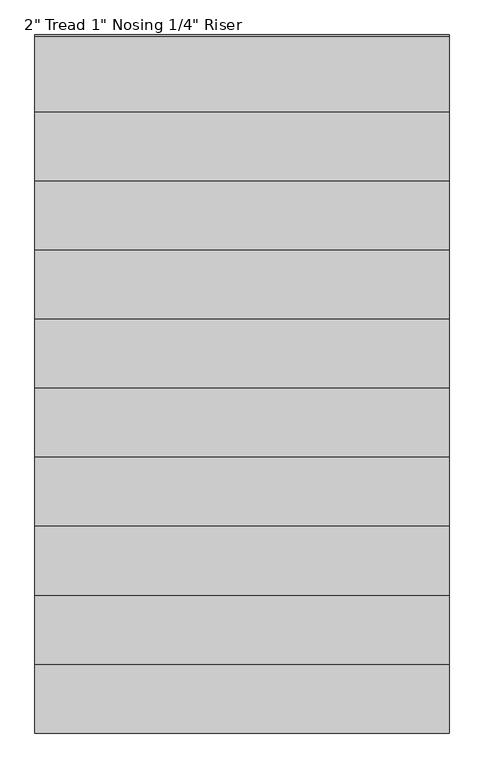
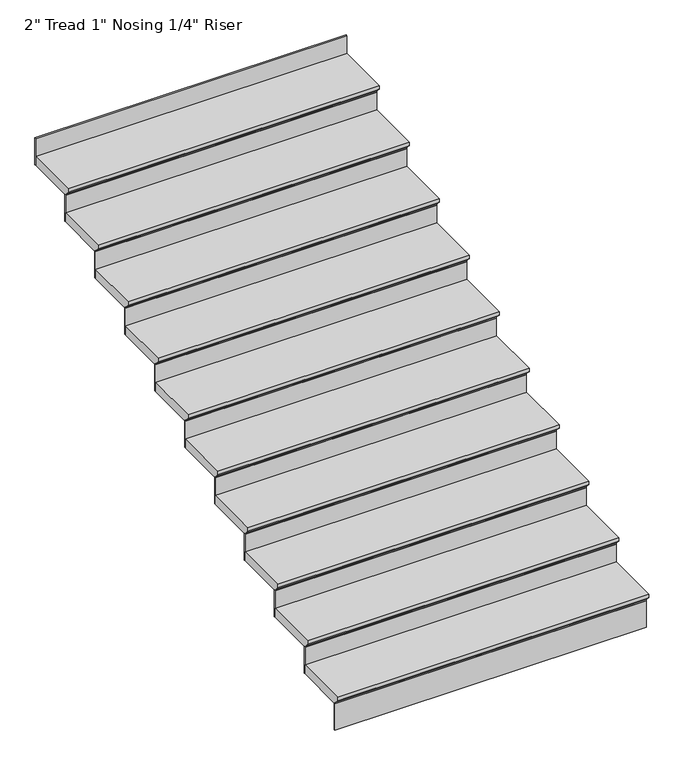
"""IFC4 building model written with IfcOpenShell, lengths in millimetres: stair flight geometry."""

from ifc_helpers import new_model, si_unit, frame, origin, place, context, project, spatial, polyline, outline, extrude, source, transform, mapped, element, save


def stair_flight_a36623a9(model_context):
    return source(origin(), model_context, "Body", "SweptSolid", [
        extrude(outline(polyline([(30952.1590238, 2286.0), (31256.9590238, 2286.0), (31256.9590238, 2235.2), (30977.5590238, 2235.2), (30977.5590238, 2241.55), (30952.1590238, 2266.95), (30952.1590238, 2286.0)])), frame((55546.5312819, 0.0, 0.0), z_axis=(1.0, 0.0, 0.0), x_axis=(0.0, 1.0, 0.0)), (0.0, 0.0, 1.0), 1676.4),
        extrude(outline(polyline([(57222.9312819, 30983.9090238), (57222.9312819, 30977.5590238), (55546.5312819, 30977.5590238), (55546.5312819, 30983.9090238), (57222.9312819, 30983.9090238)])), frame((0.0, 0.0, 2082.8), z_axis=(0.0, 0.0, 1.0), x_axis=(1.0, 0.0, 0.0)), (0.0, 0.0, 1.0), 152.4),
        extrude(outline(polyline([(57222.9312819, 31263.3090238), (57222.9312819, 31256.9590238), (55546.5312819, 31256.9590238), (55546.5312819, 31263.3090238), (57222.9312819, 31263.3090238)])), frame((0.0, 0.0, 2235.2), z_axis=(0.0, 0.0, 1.0), x_axis=(1.0, 0.0, 0.0)), (0.0, 0.0, 1.0), 152.4),
        extrude(outline(polyline([(31231.5590238, 2438.4), (31536.3590238, 2438.4), (31536.3590238, 2387.6), (31256.9590238, 2387.6), (31256.9590238, 2393.95), (31231.5590238, 2419.35), (31231.5590238, 2438.4)])), frame((55546.5312819, 0.0, 0.0), z_axis=(1.0, 0.0, 0.0), x_axis=(0.0, 1.0, 0.0)), (0.0, 0.0, 1.0), 1676.4),
        extrude(outline(polyline([(57222.9312819, 31542.7090238), (57222.9312819, 31536.3590238), (55546.5312819, 31536.3590238), (55546.5312819, 31542.7090238), (57222.9312819, 31542.7090238)])), frame((0.0, 0.0, 2387.6), z_axis=(0.0, 0.0, 1.0), x_axis=(1.0, 0.0, 0.0)), (0.0, 0.0, 1.0), 152.4),
        extrude(outline(polyline([(31510.9590238, 2590.8), (31815.7590238, 2590.8), (31815.7590238, 2540.0), (31536.3590238, 2540.0), (31536.3590238, 2546.35), (31510.9590238, 2571.75), (31510.9590238, 2590.8)])), frame((55546.5312819, 0.0, 0.0), z_axis=(1.0, 0.0, 0.0), x_axis=(0.0, 1.0, 0.0)), (0.0, 0.0, 1.0), 1676.4),
        extrude(outline(polyline([(57222.9312819, 31822.1090238), (57222.9312819, 31815.7590238), (55546.5312819, 31815.7590238), (55546.5312819, 31822.1090238), (57222.9312819, 31822.1090238)])), frame((0.0, 0.0, 2540.0), z_axis=(0.0, 0.0, 1.0), x_axis=(1.0, 0.0, 0.0)), (0.0, 0.0, 1.0), 152.4),
        extrude(outline(polyline([(31790.3590238, 2743.2), (32095.1590238, 2743.2), (32095.1590238, 2692.4), (31815.7590238, 2692.4), (31815.7590238, 2698.75), (31790.3590238, 2724.15), (31790.3590238, 2743.2)])), frame((55546.5312819, 0.0, 0.0), z_axis=(1.0, 0.0, 0.0), x_axis=(0.0, 1.0, 0.0)), (0.0, 0.0, 1.0), 1676.4),
        extrude(outline(polyline([(57222.9312819, 32101.5090238), (57222.9312819, 32095.1590238), (55546.5312819, 32095.1590238), (55546.5312819, 32101.5090238), (57222.9312819, 32101.5090238)])), frame((0.0, 0.0, 2692.4), z_axis=(0.0, 0.0, 1.0), x_axis=(1.0, 0.0, 0.0)), (0.0, 0.0, 1.0), 152.4),
        extrude(outline(polyline([(32069.7590238, 2895.6), (32374.5590238, 2895.6), (32374.5590238, 2844.8), (32095.1590238, 2844.8), (32095.1590238, 2851.15), (32069.7590238, 2876.55), (32069.7590238, 2895.6)])), frame((55546.5312819, 0.0, 0.0), z_axis=(1.0, 0.0, 0.0), x_axis=(0.0, 1.0, 0.0)), (0.0, 0.0, 1.0), 1676.4),
        extrude(outline(polyline([(57222.9312819, 32380.9090238), (57222.9312819, 32374.5590238), (55546.5312819, 32374.5590238), (55546.5312819, 32380.9090238), (57222.9312819, 32380.9090238)])), frame((0.0, 0.0, 2844.8), z_axis=(0.0, 0.0, 1.0), x_axis=(1.0, 0.0, 0.0)), (0.0, 0.0, 1.0), 152.4),
        extrude(outline(polyline([(32349.1590238, 3048.0), (32653.9590238, 3048.0), (32653.9590238, 2997.2), (32374.5590238, 2997.2), (32374.5590238, 3003.55), (32349.1590238, 3028.95), (32349.1590238, 3048.0)])), frame((55546.5312819, 0.0, 0.0), z_axis=(1.0, 0.0, 0.0), x_axis=(0.0, 1.0, 0.0)), (0.0, 0.0, 1.0), 1676.4),
        extrude(outline(polyline([(57222.9312819, 32660.3090238), (57222.9312819, 32653.9590238), (55546.5312819, 32653.9590238), (55546.5312819, 32660.3090238), (57222.9312819, 32660.3090238)])), frame((0.0, 0.0, 2997.2), z_axis=(0.0, 0.0, 1.0), x_axis=(1.0, 0.0, 0.0)), (0.0, 0.0, 1.0), 152.4),
        extrude(outline(polyline([(32628.5590238, 3200.4), (32933.3590238, 3200.4), (32933.3590238, 3149.6), (32653.9590238, 3149.6), (32653.9590238, 3155.95), (32628.5590238, 3181.35), (32628.5590238, 3200.4)])), frame((55546.5312819, 0.0, 0.0), z_axis=(1.0, 0.0, 0.0), x_axis=(0.0, 1.0, 0.0)), (0.0, 0.0, 1.0), 1676.4),
        extrude(outline(polyline([(57222.9312819, 32939.7090238), (57222.9312819, 32933.3590238), (55546.5312819, 32933.3590238), (55546.5312819, 32939.7090238), (57222.9312819, 32939.7090238)])), frame((0.0, 0.0, 3149.6), z_axis=(0.0, 0.0, 1.0), x_axis=(1.0, 0.0, 0.0)), (0.0, 0.0, 1.0), 152.4),
        extrude(outline(polyline([(32907.9590238, 3352.8), (33212.7590238, 3352.8), (33212.7590238, 3302.0), (32933.3590238, 3302.0), (32933.3590238, 3308.35), (32907.9590238, 3333.75), (32907.9590238, 3352.8)])), frame((55546.5312819, 0.0, 0.0), z_axis=(1.0, 0.0, 0.0), x_axis=(0.0, 1.0, 0.0)), (0.0, 0.0, 1.0), 1676.4),
        extrude(outline(polyline([(57222.9312819, 33219.1090238), (57222.9312819, 33212.7590238), (55546.5312819, 33212.7590238), (55546.5312819, 33219.1090238), (57222.9312819, 33219.1090238)])), frame((0.0, 0.0, 3302.0), z_axis=(0.0, 0.0, 1.0), x_axis=(1.0, 0.0, 0.0)), (0.0, 0.0, 1.0), 152.4),
        extrude(outline(polyline([(33187.3590238, 3505.2), (33492.1590238, 3505.2), (33492.1590238, 3454.4), (33212.7590238, 3454.4), (33212.7590238, 3460.75), (33187.3590238, 3486.15), (33187.3590238, 3505.2)])), frame((55546.5312819, 0.0, 0.0), z_axis=(1.0, 0.0, 0.0), x_axis=(0.0, 1.0, 0.0)), (0.0, 0.0, 1.0), 1676.4),
        extrude(outline(polyline([(57222.9312819, 33498.5090238), (57222.9312819, 33492.1590238), (55546.5312819, 33492.1590238), (55546.5312819, 33498.5090238), (57222.9312819, 33498.5090238)])), frame((0.0, 0.0, 3454.4), z_axis=(0.0, 0.0, 1.0), x_axis=(1.0, 0.0, 0.0)), (0.0, 0.0, 1.0), 152.4),
        extrude(outline(polyline([(57222.9312819, 33777.9090238), (57222.9312819, 33771.5590238), (55546.5312819, 33771.5590238), (55546.5312819, 33777.9090238), (57222.9312819, 33777.9090238)])), frame((0.0, 0.0, 3606.8), z_axis=(0.0, 0.0, 1.0), x_axis=(1.0, 0.0, 0.0)), (0.0, 0.0, 1.0), 152.4),
        extrude(outline(polyline([(33466.7590238, 3657.6), (33771.5590238, 3657.6), (33771.5590238, 3606.8), (33492.1590238, 3606.8), (33492.1590238, 3613.15), (33466.7590238, 3638.55), (33466.7590238, 3657.6)])), frame((55546.5312819, 0.0, 0.0), z_axis=(1.0, 0.0, 0.0), x_axis=(0.0, 1.0, 0.0)), (0.0, 0.0, 1.0), 1676.4),
    ])


if __name__ == "__main__":
    model = new_model("IFC4")
    model_context = context("Model", 3, world=origin())
    ifc_project = project(units=[si_unit("LENGTHUNIT", "METRE", prefix="MILLI")], contexts=[model_context])
    site = spatial("IfcSite", under=ifc_project)
    building = spatial("IfcBuilding", under=site)
    placement = place(None, origin())
    stair_flight_shape = stair_flight_a36623a9(model_context)
    element("IfcStairFlight", 1, ObjectType="2\" Tread 1\" Nosing 1/4\" Riser", at=placement, inside=building, context=model_context, shape_type="MappedRepresentation", body=[
        mapped(stair_flight_shape, transform((0.0, 0.0, 0.0), x_axis=(1.0, 0.0, 0.0), y_axis=(0.0, 1.0, 0.0), z_axis=(0.0, 0.0, 1.0))),
    ])
    save(model, "model.ifc")
